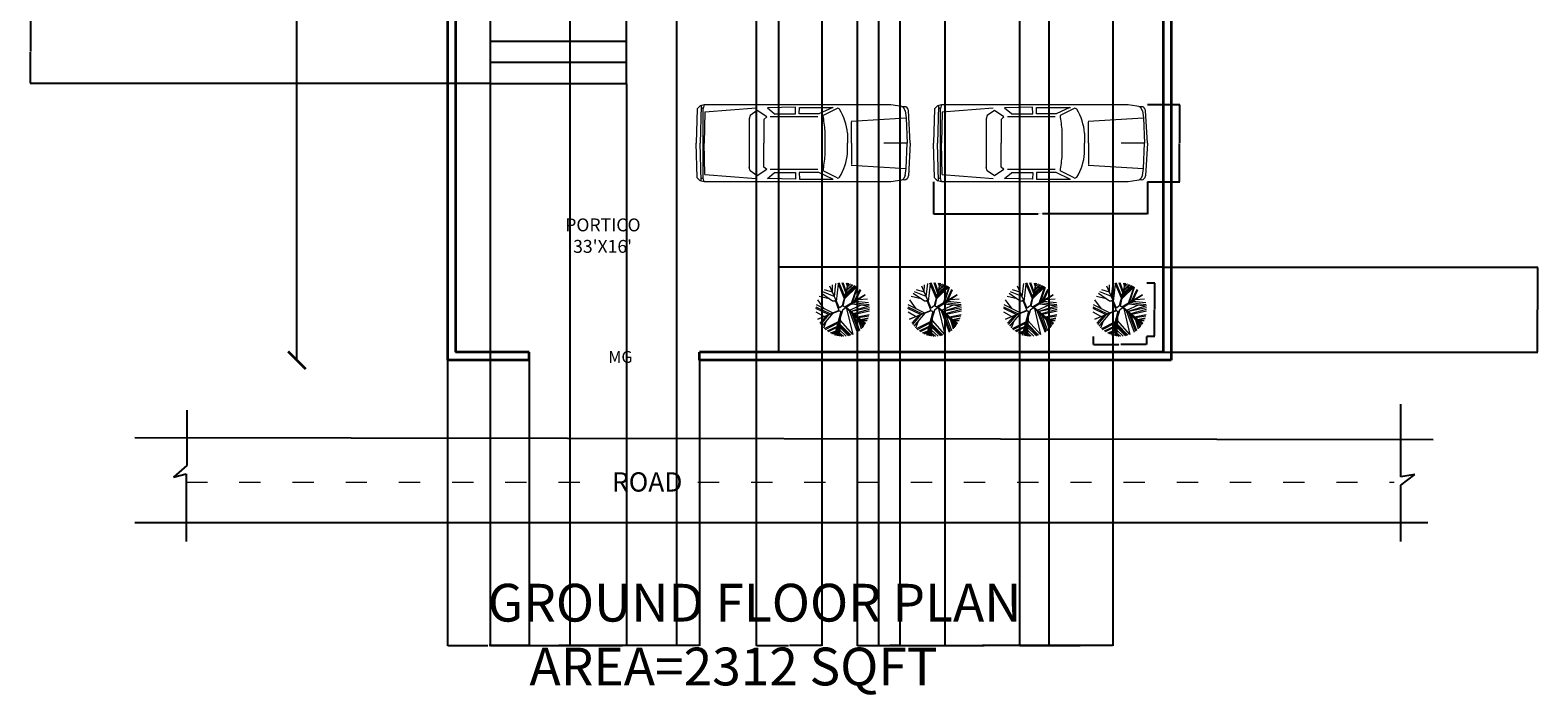
# Model space of a CAD drawing. Units: inches. Extents: x 338 to 1188, y -996 to 127.
# Tile 1 of 15: x 338 to 1188, y -996 to -622. Entities that reach past the tile are written whole.
import ezdxf

# ---------------------------------------------------------------- set-up
doc = ezdxf.new("R2010")
doc.units = ezdxf.units.IN
doc.header["$MEASUREMENT"] = 0
doc.linetypes.add('ACAD_ISO03W100', pattern=[30, 12, -18])
for name, color, linetype, lineweight in [('A-ANNO-DIMS', 5, 'Continuous', 18), ('A-ANNO-TEXT', 7, 'Continuous', 18), ('A-ANNO-TITL', 7, 'Continuous', 35), ('A-AREA-IDEN', 8, 'Continuous', 18), ('A-FLOR-STRS', 7, 'Continuous', 25), ('C-PKNG-VEHI', 8, 'Continuous', 18), ('C-PROP', 1, 'Continuous', 35), ('C-ROAD', 7, 'Continuous', 25), ('C-ROAD-MRKG', 7, 'ACAD_ISO03W100', 18), ('L-PLNT-BEDS', 90, 'Continuous', 25)]:
    doc.layers.add(name, color=color, linetype=linetype, lineweight=lineweight)
doc.layers.add('GRASS', color=90, linetype='Continuous', lineweight=18, transparency=0.7)
doc.styles.get("Standard").update_dxf_attribs({"font": 'arial.ttf'})
doc.dimstyles.get("Standard").update_dxf_attribs({"dimtxt": 0.18, "dimasz": 0.18, "dimexe": 0.18, "dimexo": 0.0625, "dimgap": 0.09, "dimtad": 0, "dimtih": 1, "dimtoh": 1, "dimdec": 1, "dimzin": 0, "dimdsep": 46, "dimlunit": 4, "dimtxsty": 'Standard', "dimcen": 0.09, "dimadec": 0, "dimazin": 0, "dimtfac": 1, "dimtdec": 1, "dimtofl": 0, "dimtmove": 0, "dimatfit": 3, "dimfxl": 1, "dimtolj": 1, "dimtzin": 0, "dimarcsym": 0})

# ---------------------------------------------------------------- blocks, each defined once
blk = doc.blocks.new('A$C4FA53466')
at = {"color": 0}
for p, q in [((0.505, 1.347), (0.266, 1.426)), ((0.717, 0.864), (0.422, 1.538)), ((0.501, 1.356), (0.505, 1.578)), ((0.563, 1.216), (0.612, 1.614)), ((0.627, 1.07), (0.687, 1.601)), ((0.867, 1.166), (0.675, 1.628)), ((0.882, 1.223), (0.709, 1.633)), ((0.91, 1.328), (0.802, 1.64)), ((0.988, 1.623), (0.804, 0.931)), ((0.925, 1.384), (0.834, 1.64)), ((0.836, 0.927), (0.988, 1.623)), ((0.887, 1.159), (1.256, 1.515)), ((0.901, 1.223), (1.228, 1.532)), ((0.914, 1.283), (1.197, 1.549)), ((0.922, 1.323), (1.176, 1.559)), ((0.964, 1.534), (0.938, 1.632)), ((0.938, 1.393), (1.132, 1.579)), ((0.945, 1.425), (1.104, 1.59)), ((0.967, 1.545), (0.952, 1.63)), ((0.965, 1.517), (1.059, 1.605)), ((0.974, 1.559), (1.002, 1.62)), ((1.085, 1.015), (1.262, 1.512)), ((1.121, 1.036), (1.274, 1.503)), ((1.18, 1.071), (1.349, 1.447)), ((1.222, 1.096), (1.37, 1.428)), ((0.501, 0.716), (0.012, 0.965)), ((0.255, 0.841), (0.055, 1.116)), ((0.406, 1.148), (0.102, 1.217)), ((0.506, 1.079), (0.165, 1.314)), ((0.562, 1.217), (0.205, 1.363)), ((0.614, 1.092), (0.506, 1.079)), ((0.604, 1.069), (0.506, 1.079)), ((0.715, 0.784), (0.604, 1.069)), ((0.804, 0.931), (0.717, 0.864)), ((0.879, 0.894), (0.836, 0.927)), ((1.509, 1.265), (0.879, 0.894)), ((0.926, 0.889), (1.509, 1.265)), ((1.03, 0.802), (1.392, 0.963)), ((1.073, 0.767), (1.614, 0.936)), ((1.097, 0.999), (1.632, 0.934)), ((1.148, 1.032), (1.626, 0.972)), ((1.211, 1.073), (1.612, 1.034)), ((1.3, 1.13), (1.573, 1.147)), ((0.384, 0.667), (0, 0.848)), ((0.436, 0.689), (0.003, 0.892)), ((0.237, 0.605), (0.004, 0.735)), ((0.053, 0.528), (0.708, 0.803)), ((0.716, 0.781), (0.053, 0.528)), ((0.321, 0.63), (0.115, 0.4)), ((0.387, 0.655), (0.137, 0.366)), ((0.516, 0.704), (0.179, 0.309)), ((0.313, 0.466), (0.232, 0.248)), ((0.82, 0.82), (0.575, 0.037)), ((0.575, 0.037), (0.769, 0.772)), ((0.732, 0.539), (0.664, 0.015)), ((0.737, 0.554), (0.691, 0.01)), ((0.715, 0.784), (0.775, 0.767)), ((0.744, 0.569), (0.717, 0.006)), ((0.74, 0.488), (1.121, 0.057)), ((0.82, 0.82), (0.904, 0.875)), ((1.521, 0.394), (0.904, 0.875)), ((0.926, 0.889), (1.521, 0.394)), ((0.938, 0.848), (1.126, 0.059)), ((1.016, 0.788), (1.263, 0.13)), ((1.04, 0.769), (1.475, 0.326)), ((1.06, 0.754), (1.5, 0.362)), ((1.081, 0.769), (1.638, 0.886)), ((1.083, 0.725), (1.298, 0.153)), ((1.153, 0.701), (1.64, 0.826)), ((1.161, 0.646), (1.335, 0.182)), ((1.185, 0.674), (1.639, 0.776)), ((1.273, 0.601), (1.627, 0.672)), ((1.298, 0.58), (1.618, 0.629)), ((1.301, 0.503), (1.386, 0.227)), ((1.376, 0.515), (1.599, 0.562)), ((1.392, 0.502), (1.593, 0.545)), ((1.412, 0.486), (1.569, 0.486)), ((0.682, 0.44), (0.255, 0.225)), ((0.673, 0.407), (0.281, 0.201)), ((0.645, 0.301), (0.342, 0.153)), ((0.636, 0.267), (0.375, 0.133)), ((0.608, 0.161), (0.439, 0.093)), ((0.6, 0.133), (0.475, 0.076)), ((0.59, 0.094), (0.501, 0.064)), ((0.701, 0.44), (0.621, 0.024)), ((0.72, 0.07), (0.793, 0)), ((0.722, 0.111), (0.842, 0)), ((0.726, 0.192), (0.924, 0.006)), ((0.73, 0.277), (0.998, 0.019)), ((0.733, 0.326), (1.037, 0.029)), ((0.735, 0.369), (1.067, 0.038)), ((1.365, 0.438), (1.42, 0.26)), ((1.413, 0.39), (1.444, 0.288))]:
    blk.add_line(p, q, dxfattribs=at)
blk = doc.blocks.new('02PCAR12')
at = {"color": 0, "linetype": 'ByBlock'}
for p, q in [((-210, 34), (-211, 0)), ((-207, 37), (-210, 34)), ((-203, 38), (-207, 37)), ((-206, 37), (-207, 0)), ((-204, 34.1), (-206, 35.1)), ((-203, 38.1), (-204, 34.1)), ((-204, -34), (-204, 34)), ((-19, 38), (-203, 38)), ((-202.4, 30.8), (-203, 0)), ((-202.4, 30.8), (-152, 35)), ((-150.8, 32.3), (-157.9, 27.3)), ((-141.5, 26), (-150.8, 32.3)), ((-113.2, 35.5), (-140.8, 34.9)), ((-140.8, 34.9), (-134, 29.2)), ((-113, 29), (-113.2, 35.5)), ((-109.4, 29), (-109.2, 35.3)), ((-109.2, 35.3), (-75.9, 35.3)), ((-76.4, 35.3), (-90, 29)), ((-72.1, 34.2), (-85.9, 27.4)), ((-6, 36), (-19, 38)), ((-5, 32), (-6.4, 34.9)), ((-5, 32), (-4, 25)), ((0, 0), (-1.8, 32.2)), ((-157.9, 27.3), (-158.9, 24.1)), ((-158.9, 24.1), (-158.9, -24)), ((-141.5, 26), (-144.2, 23.5)), ((-144.2, 23.5), (-144.2, 0)), ((-91, 26), (-138, 26)), ((-134, 29), (-113, 29)), ((-90, 29), (-109.4, 29)), ((-58.3, 21.8), (-4, 25)), ((-58, 0), (-58, 21)), ((-4, 25), (-3, 0)), ((-210, -34), (-211, 0)), ((-206, -37), (-207, 0)), ((-202.4, -30.8), (-203, 0)), ((-144.2, -23.5), (-144.2, 0)), ((-84, -12), (-84, 12)), ((-62, 10), (-62, 0)), ((-62, -10), (-62, 0)), ((-58, 0), (-58, -21)), ((-3, 0), (-26, 0)), ((-4, -25), (-3, 0)), ((0, 0), (-1.8, -32.2)), ((-157.9, -27.3), (-158.9, -24.1)), ((-150.8, -32.3), (-157.9, -27.3)), ((-141.5, -26), (-150.8, -32.3)), ((-141.5, -26), (-144.2, -23.5)), ((-140.8, -34.9), (-134, -29.2)), ((-91, -26), (-138, -26)), ((-134, -29), (-113, -29)), ((-113, -29), (-113.2, -35.5)), ((-90, -29), (-109.4, -29)), ((-109.4, -29), (-109.2, -35.3)), ((-76.4, -35.3), (-90, -29)), ((-72.1, -34.2), (-85.9, -27.4)), ((-58.3, -21.8), (-4, -25)), ((-5, -32), (-4, -25)), ((-207, -37), (-210, -34)), ((-203, -38), (-207, -37)), ((-204, -34), (-206, -35)), ((-203, -38), (-204, -34)), ((-19, -38), (-203, -38)), ((-202.4, -30.7), (-152, -34.9)), ((-113.2, -35.5), (-140.8, -34.9)), ((-109.2, -35.3), (-75.9, -35.3)), ((-6, -36), (-19, -38)), ((-5, -32), (-6.4, -34.9))]:
    blk.add_line(p, q, dxfattribs=at)
for centre, radius, start, end in [((-71.4, 32.4), 2, 31.5638, 113.1257), ((-115.3, 5.4), 53.6, 4.9379, 31.5638), ((-8.2, 34), 2, 26.5651, 90), ((-5.8, 32), 4, 3.0128, 90), ((-461, -27.1), 379.1, 5.9264, 8.267), ((-461, 27.1), 379.1, 351.733, 354.0736), ((-115.3, -5.4), 53.6, 328.4362, 355.0621), ((-71.4, -32.4), 2, 246.8743, 328.4362), ((-8.2, -34), 2, 270, 333.4349), ((-5.8, -32), 4, 270, 356.9872)]:
    blk.add_arc(centre, radius, start, end, dxfattribs=at)
blk = doc.blocks.new('_ArchTick')
at = {"color": 0, "linetype": 'ByBlock', "const_width": 0.15}
blk.add_lwpolyline([(-0.5, -0.5), (0.5, 0.5)], dxfattribs=at)
blk = doc.blocks.new('*D7')
at = {"layer": 'A-ANNO-DIMS', "color": 0, "lineweight": -2, "transparency": 16777216}
for p, q in [((488.01, 8.27), (488.01, -388.07)), ((488.01, -807.73), (488.01, -411.39))]:
    blk.add_line(p, q, dxfattribs=at)
at = {"layer": 'Defpoints', "color": 0, "transparency": 16777216}
for p in [(572.96, 8.27), (488.01, -807.73), (572.96, -807.73)]:
    blk.add_point(p, dxfattribs=at)
at = {"layer": 'A-ANNO-DIMS', "color": 0, "lineweight": -2, "transparency": 16777216, "xscale": 10, "yscale": 10, "zscale": 10}
for p, rotation in [((488.01, 8.27), 90), ((488.01, -807.73), 270)]:
    blk.add_blockref('_ArchTick', p, dxfattribs=dict(at, rotation=rotation))
at = {"layer": 'A-ANNO-DIMS', "color": 0, "transparency": 16777216, "insert": (488.01, -399.73), "char_height": 9, "attachment_point": 5, "rotation": 90}
blk.add_mtext("\\A1;68'", dxfattribs=at)
blk = doc.blocks.new('*D11')
at = {"layer": 'A-ANNO-DIMS', "color": 0, "lineweight": -2, "transparency": 16777216}
for p, q in [((967.16, -764.04), (971.81, -764.04)), ((971.63, -764.22), (971.63, -778.96)), ((971.63, -794.07), (971.63, -779.33)), ((967.16, -794.25), (971.81, -794.25))]:
    blk.add_line(p, q, dxfattribs=at)
at = {"layer": 'A-ANNO-DIMS', "color": 0, "transparency": 16777216}
for points in [[(971.6, -764.22), (971.66, -764.22), (971.63, -764.04)], [(971.6, -794.07), (971.66, -794.07), (971.63, -794.25)]]:
    blk.add_solid(points, dxfattribs=at)
at = {"layer": 'Defpoints', "color": 0, "transparency": 16777216}
for p in [(967.1, -764.04), (971.63, -764.04), (967.1, -794.25)]:
    blk.add_point(p, dxfattribs=at)
at = {"layer": 'A-ANNO-DIMS', "color": 0, "transparency": 16777216, "insert": (971.63, -779.14), "char_height": 0.18, "attachment_point": 5}
blk.add_mtext('\\A1;SHRUB 2\'-6" TYP.', dxfattribs=at)
blk = doc.blocks.new('*D12')
at = {"layer": 'A-ANNO-DIMS', "color": 0, "lineweight": -2, "transparency": 16777216}
for p, q in [((936.89, -794.31), (936.89, -798.96)), ((937.07, -798.78), (951.36, -798.78)), ((966.92, -798.78), (952.64, -798.78)), ((967.1, -794.31), (967.1, -798.96))]:
    blk.add_line(p, q, dxfattribs=at)
at = {"layer": 'A-ANNO-DIMS', "color": 0, "transparency": 16777216}
for points in [[(937.07, -798.75), (937.07, -798.81), (936.89, -798.78)], [(966.92, -798.75), (966.92, -798.81), (967.1, -798.78)]]:
    blk.add_solid(points, dxfattribs=at)
at = {"layer": 'Defpoints', "color": 0, "transparency": 16777216}
for p in [(936.89, -794.25), (967.1, -794.25), (967.1, -798.78)]:
    blk.add_point(p, dxfattribs=at)
at = {"layer": 'A-ANNO-DIMS', "color": 0, "transparency": 16777216, "insert": (952, -798.78), "char_height": 0.18, "attachment_point": 5}
blk.add_mtext('\\A1;2\'-6" TYP.', dxfattribs=at)
blk = doc.blocks.new('*D13')
at = {"layer": 'A-ANNO-DIMS', "color": 0, "lineweight": -2, "transparency": 16777216}
for p, q in [((846.88, -707.14), (846.88, -725.36)), ((967.54, -707.14), (967.54, -725.36)), ((847.06, -725.18), (905.99, -725.18)), ((967.36, -725.18), (908.43, -725.18))]:
    blk.add_line(p, q, dxfattribs=at)
at = {"layer": 'A-ANNO-DIMS', "color": 0, "transparency": 16777216}
for points in [[(847.06, -725.15), (847.06, -725.21), (846.88, -725.18)], [(967.36, -725.15), (967.36, -725.21), (967.54, -725.18)]]:
    blk.add_solid(points, dxfattribs=at)
at = {"layer": 'Defpoints', "color": 0, "transparency": 16777216}
for p in [(846.88, -707.08), (967.54, -707.08), (967.54, -725.18)]:
    blk.add_point(p, dxfattribs=at)
at = {"layer": 'A-ANNO-DIMS', "color": 0, "transparency": 16777216, "insert": (907.21, -725.18), "char_height": 0.18, "attachment_point": 5}
blk.add_mtext('\\A1;CAR 10\'-0 1/2" TYP.', dxfattribs=at)
blk = doc.blocks.new('*D14')
at = {"layer": 'A-ANNO-DIMS', "color": 0, "lineweight": -2, "transparency": 16777216}
for p, q in [((967.6, -663.57), (985.82, -663.57)), ((985.64, -663.75), (985.64, -685.14)), ((985.64, -706.9), (985.64, -685.51)), ((967.6, -707.08), (985.82, -707.08))]:
    blk.add_line(p, q, dxfattribs=at)
at = {"layer": 'A-ANNO-DIMS', "color": 0, "transparency": 16777216}
for points in [[(985.61, -663.75), (985.67, -663.75), (985.64, -663.57)], [(985.61, -706.9), (985.67, -706.9), (985.64, -707.08)]]:
    blk.add_solid(points, dxfattribs=at)
at = {"layer": 'Defpoints', "color": 0, "transparency": 16777216}
for p in [(967.54, -663.57), (985.64, -663.57), (967.54, -707.08)]:
    blk.add_point(p, dxfattribs=at)
at = {"layer": 'A-ANNO-DIMS', "color": 0, "transparency": 16777216, "insert": (985.64, -685.32), "char_height": 0.18, "attachment_point": 5}
blk.add_mtext('\\A1;3\'-7 1/2" TYP.', dxfattribs=at)
blk = doc.blocks.new('*D21')
at = {"layer": 'A-ANNO-DIMS', "color": 0, "lineweight": -2, "transparency": 16777216}
for p, q in [((618.97, -807.8), (618.97, -968.86)), ((714.97, -807.8), (714.97, -968.86)), ((619.15, -968.68), (666.64, -968.68)), ((714.79, -968.68), (667.3, -968.68))]:
    blk.add_line(p, q, dxfattribs=at)
at = {"layer": 'A-ANNO-DIMS', "color": 0, "transparency": 16777216}
for points in [[(619.15, -968.65), (619.15, -968.71), (618.97, -968.68)], [(714.79, -968.65), (714.79, -968.71), (714.97, -968.68)]]:
    blk.add_solid(points, dxfattribs=at)
at = {"layer": 'Defpoints', "color": 0, "transparency": 16777216}
for p in [(618.97, -807.73), (714.97, -807.73), (714.97, -968.68)]:
    blk.add_point(p, dxfattribs=at)
at = {"layer": 'A-ANNO-DIMS', "color": 0, "transparency": 16777216, "insert": (666.97, -968.68), "char_height": 0.18, "attachment_point": 5}
blk.add_mtext('\\A1;8\'-0"', dxfattribs=at)
blk = doc.blocks.new('*D22')
at = {"layer": 'A-ANNO-DIMS', "color": 0, "lineweight": -2, "transparency": 16777216}
for p, q in [((596.9, -615.73), (337.66, -615.73)), ((337.84, -615.91), (337.84, -633.55)), ((337.84, -651.55), (337.84, -633.92)), ((596.9, -651.73), (337.66, -651.73))]:
    blk.add_line(p, q, dxfattribs=at)
at = {"layer": 'A-ANNO-DIMS', "color": 0, "transparency": 16777216}
for points in [[(337.81, -615.91), (337.87, -615.91), (337.84, -615.73)], [(337.81, -651.55), (337.87, -651.55), (337.84, -651.73)]]:
    blk.add_solid(points, dxfattribs=at)
at = {"layer": 'Defpoints', "color": 0, "transparency": 16777216}
for p in [(596.96, -615.73), (337.84, -651.73), (596.96, -651.73)]:
    blk.add_point(p, dxfattribs=at)
at = {"layer": 'A-ANNO-DIMS', "color": 0, "transparency": 16777216, "insert": (337.84, -633.73), "char_height": 0.18, "attachment_point": 5}
blk.add_mtext('\\A1;3\'-0"', dxfattribs=at)
blk = doc.blocks.new('*D23')
at = {"layer": 'A-ANNO-DIMS', "color": 0, "lineweight": -2, "transparency": 16777216}
for p, q in [((596.96, -651.8), (596.96, -968.86)), ((673.79, -651.8), (673.79, -968.86)), ((597.14, -968.68), (635.05, -968.68)), ((673.61, -968.68), (635.71, -968.68))]:
    blk.add_line(p, q, dxfattribs=at)
at = {"layer": 'A-ANNO-DIMS', "color": 0, "transparency": 16777216}
for points in [[(597.14, -968.65), (597.14, -968.71), (596.96, -968.68)], [(673.61, -968.65), (673.61, -968.71), (673.79, -968.68)]]:
    blk.add_solid(points, dxfattribs=at)
at = {"layer": 'Defpoints', "color": 0, "transparency": 16777216}
for p in [(596.96, -651.73), (673.79, -651.73), (673.79, -968.68)]:
    blk.add_point(p, dxfattribs=at)
at = {"layer": 'A-ANNO-DIMS', "color": 0, "transparency": 16777216, "insert": (635.38, -968.68), "char_height": 0.18, "attachment_point": 5}
blk.add_mtext('\\A1;6\'-5"', dxfattribs=at)
blk = doc.blocks.new('*D26')
at = {"layer": 'A-ANNO-DIMS', "color": 0, "lineweight": -2, "transparency": 16777216}
for p, q in [((815.96, -297.8), (815.96, -968.86)), ((827.96, -297.8), (827.96, -968.86)), ((816.14, -968.68), (821.64, -968.68)), ((827.78, -968.68), (822.28, -968.68))]:
    blk.add_line(p, q, dxfattribs=at)
at = {"layer": 'A-ANNO-DIMS', "color": 0, "transparency": 16777216}
for points in [[(816.14, -968.65), (816.14, -968.71), (815.96, -968.68)], [(827.78, -968.65), (827.78, -968.71), (827.96, -968.68)]]:
    blk.add_solid(points, dxfattribs=at)
at = {"layer": 'Defpoints', "color": 0, "transparency": 16777216}
for p in [(815.96, -297.73), (827.96, -297.73), (827.96, -968.68)]:
    blk.add_point(p, dxfattribs=at)
at = {"layer": 'A-ANNO-DIMS', "color": 0, "transparency": 16777216, "insert": (821.96, -968.68), "char_height": 0.18, "attachment_point": 5}
blk.add_mtext('\\A1;1\'-0"', dxfattribs=at)
blk = doc.blocks.new('*D27')
at = {"layer": 'A-ANNO-DIMS', "color": 0, "lineweight": -2, "transparency": 16777216}
for p, q in [((911.96, -297.8), (911.96, -968.86)), ((947.96, -297.8), (947.96, -968.86)), ((912.14, -968.68), (929.63, -968.68)), ((947.78, -968.68), (930.29, -968.68))]:
    blk.add_line(p, q, dxfattribs=at)
at = {"layer": 'A-ANNO-DIMS', "color": 0, "transparency": 16777216}
for points in [[(912.14, -968.65), (912.14, -968.71), (911.96, -968.68)], [(947.78, -968.65), (947.78, -968.71), (947.96, -968.68)]]:
    blk.add_solid(points, dxfattribs=at)
at = {"layer": 'Defpoints', "color": 0, "transparency": 16777216}
for p in [(911.96, -297.73), (947.96, -297.73), (947.96, -968.68)]:
    blk.add_point(p, dxfattribs=at)
at = {"layer": 'A-ANNO-DIMS', "color": 0, "transparency": 16777216, "insert": (929.96, -968.68), "char_height": 0.18, "attachment_point": 5}
blk.add_mtext('\\A1;3\'-0"', dxfattribs=at)
blk = doc.blocks.new('*D28')
at = {"layer": 'A-ANNO-DIMS', "color": 0, "lineweight": -2, "transparency": 16777216}
for p, q in [((803.96, -265.8), (803.96, -968.86)), ((947.96, -297.8), (947.96, -968.86)), ((804.14, -968.68), (875.57, -968.68)), ((947.78, -968.68), (876.35, -968.68))]:
    blk.add_line(p, q, dxfattribs=at)
at = {"layer": 'A-ANNO-DIMS', "color": 0, "transparency": 16777216}
for points in [[(804.14, -968.65), (804.14, -968.71), (803.96, -968.68)], [(947.78, -968.65), (947.78, -968.71), (947.96, -968.68)]]:
    blk.add_solid(points, dxfattribs=at)
at = {"layer": 'Defpoints', "color": 0, "transparency": 16777216}
for p in [(803.96, -265.73), (947.96, -297.73), (947.96, -968.68)]:
    blk.add_point(p, dxfattribs=at)
at = {"layer": 'A-ANNO-DIMS', "color": 0, "transparency": 16777216, "insert": (875.96, -968.68), "char_height": 0.18, "attachment_point": 5}
blk.add_mtext('\\A1;12\'-0"', dxfattribs=at)
blk = doc.blocks.new('*D31')
at = {"layer": 'A-ANNO-DIMS', "color": 0, "lineweight": -2, "transparency": 16777216}
for p, q in [((641.96, -149.3), (641.96, -968.86)), ((701.96, -149.3), (701.96, -968.86)), ((642.14, -968.68), (671.63, -968.68)), ((701.78, -968.68), (672.29, -968.68))]:
    blk.add_line(p, q, dxfattribs=at)
at = {"layer": 'A-ANNO-DIMS', "color": 0, "transparency": 16777216}
for points in [[(642.14, -968.65), (642.14, -968.71), (641.96, -968.68)], [(701.78, -968.65), (701.78, -968.71), (701.96, -968.68)]]:
    blk.add_solid(points, dxfattribs=at)
at = {"layer": 'Defpoints', "color": 0, "transparency": 16777216}
for p in [(641.96, -149.23), (701.96, -149.23), (701.96, -968.68)]:
    blk.add_point(p, dxfattribs=at)
at = {"layer": 'A-ANNO-DIMS', "color": 0, "transparency": 16777216, "insert": (671.96, -968.68), "char_height": 0.18, "attachment_point": 5}
blk.add_mtext('\\A1;5\'-0"', dxfattribs=at)
blk = doc.blocks.new('*D35')
at = {"layer": 'A-ANNO-DIMS', "color": 0, "lineweight": -2, "transparency": 16777216}
for p, q in [((572.96, -807.8), (572.96, -968.86)), ((618.97, -807.8), (618.97, -968.86)), ((573.14, -968.68), (595.57, -968.68)), ((618.79, -968.68), (596.37, -968.68))]:
    blk.add_line(p, q, dxfattribs=at)
at = {"layer": 'A-ANNO-DIMS', "color": 0, "transparency": 16777216}
for points in [[(573.14, -968.65), (573.14, -968.71), (572.96, -968.68)], [(618.79, -968.65), (618.79, -968.71), (618.97, -968.68)]]:
    blk.add_solid(points, dxfattribs=at)
at = {"layer": 'Defpoints', "color": 0, "transparency": 16777216}
for p in [(572.96, -807.73), (618.97, -807.73), (618.97, -968.68)]:
    blk.add_point(p, dxfattribs=at)
at = {"layer": 'A-ANNO-DIMS', "color": 0, "transparency": 16777216, "insert": (595.97, -968.68), "char_height": 0.18, "attachment_point": 5}
blk.add_mtext('\\A1;3\'-10"', dxfattribs=at)
blk = doc.blocks.new('*D36')
at = {"layer": 'A-ANNO-DIMS', "color": 0, "lineweight": -2, "transparency": 16777216}
for p, q in [((976.53, -755.23), (1187.6, -755.23)), ((1187.42, -755.41), (1187.42, -779.05)), ((1187.42, -803.05), (1187.42, -779.41)), ((976.53, -803.23), (1187.6, -803.23))]:
    blk.add_line(p, q, dxfattribs=at)
at = {"layer": 'A-ANNO-DIMS', "color": 0, "transparency": 16777216}
for points in [[(1187.39, -755.41), (1187.45, -755.41), (1187.42, -755.23)], [(1187.39, -803.05), (1187.45, -803.05), (1187.42, -803.23)]]:
    blk.add_solid(points, dxfattribs=at)
at = {"layer": 'Defpoints', "color": 0, "transparency": 16777216}
for p in [(976.46, -755.23), (976.46, -803.23), (1187.42, -803.23)]:
    blk.add_point(p, dxfattribs=at)
at = {"layer": 'A-ANNO-DIMS', "color": 0, "transparency": 16777216, "insert": (1187.42, -779.23), "char_height": 0.18, "attachment_point": 5}
blk.add_mtext('\\A1;4\'-0"', dxfattribs=at)
blk = doc.blocks.new('*D42')
at = {"layer": 'A-ANNO-DIMS', "color": 0, "lineweight": -2, "transparency": 16777216}
for p, q in [((746.96, -54.8), (746.96, -968.86)), ((783.89, -54.8), (783.89, -968.86)), ((747.14, -968.68), (765.1, -968.68)), ((783.71, -968.68), (765.76, -968.68))]:
    blk.add_line(p, q, dxfattribs=at)
at = {"layer": 'A-ANNO-DIMS', "color": 0, "transparency": 16777216}
for points in [[(747.14, -968.65), (747.14, -968.71), (746.96, -968.68)], [(783.71, -968.65), (783.71, -968.71), (783.89, -968.68)]]:
    blk.add_solid(points, dxfattribs=at)
at = {"layer": 'Defpoints', "color": 0, "transparency": 16777216}
for p in [(746.96, -54.73), (783.89, -54.73), (783.89, -968.68)]:
    blk.add_point(p, dxfattribs=at)
at = {"layer": 'A-ANNO-DIMS', "color": 0, "transparency": 16777216, "insert": (765.43, -968.68), "char_height": 0.18, "attachment_point": 5}
blk.add_mtext('\\A1;3\'-1"', dxfattribs=at)
blk = doc.blocks.new('*D43')
at = {"layer": 'A-ANNO-DIMS', "color": 0, "lineweight": -2, "transparency": 16777216}
for p, q in [((853.28, -53.93), (853.28, -968.86)), ((895.37, -53.93), (895.37, -968.86)), ((853.46, -968.68), (873.99, -968.68)), ((895.19, -968.68), (874.65, -968.68))]:
    blk.add_line(p, q, dxfattribs=at)
at = {"layer": 'A-ANNO-DIMS', "color": 0, "transparency": 16777216}
for points in [[(853.46, -968.65), (853.46, -968.71), (853.28, -968.68)], [(895.19, -968.65), (895.19, -968.71), (895.37, -968.68)]]:
    blk.add_solid(points, dxfattribs=at)
at = {"layer": 'Defpoints', "color": 0, "transparency": 16777216}
for p in [(853.28, -53.87), (895.37, -53.87), (895.37, -968.68)]:
    blk.add_point(p, dxfattribs=at)
at = {"layer": 'A-ANNO-DIMS', "color": 0, "transparency": 16777216, "insert": (874.32, -968.68), "char_height": 0.18, "attachment_point": 5}
blk.add_mtext('\\A1;3\'-6"', dxfattribs=at)
blk = doc.blocks.new('*D44')
at = {"layer": 'A-ANNO-DIMS', "color": 0, "lineweight": -2, "transparency": 16777216}
for p, q in [((895.37, -53.93), (895.37, -968.86)), ((947.96, -54.8), (947.96, -968.86)), ((895.55, -968.68), (921.12, -968.68)), ((947.78, -968.68), (922.21, -968.68))]:
    blk.add_line(p, q, dxfattribs=at)
at = {"layer": 'A-ANNO-DIMS', "color": 0, "transparency": 16777216}
for points in [[(895.55, -968.65), (895.55, -968.71), (895.37, -968.68)], [(947.78, -968.65), (947.78, -968.71), (947.96, -968.68)]]:
    blk.add_solid(points, dxfattribs=at)
at = {"layer": 'Defpoints', "color": 0, "transparency": 16777216}
for p in [(895.37, -53.87), (947.96, -54.73), (947.96, -968.68)]:
    blk.add_point(p, dxfattribs=at)
at = {"layer": 'A-ANNO-DIMS', "color": 0, "transparency": 16777216, "insert": (921.67, -968.68), "char_height": 0.18, "attachment_point": 5}
blk.add_mtext('\\A1;4\'-4 1/2"', dxfattribs=at)
blk = doc.blocks.new('*D47')
at = {"layer": 'A-ANNO-DIMS', "color": 0, "lineweight": -2, "transparency": 16777216}
for p, q in [((759.67, -755.17), (759.67, 67.25)), ((759.85, 67.07), (867.68, 67.07)), ((976.28, 67.07), (868.46, 67.07)), ((976.46, -755.17), (976.46, 67.25))]:
    blk.add_line(p, q, dxfattribs=at)
at = {"layer": 'A-ANNO-DIMS', "color": 0, "transparency": 16777216}
for points in [[(759.85, 67.1), (759.85, 67.04), (759.67, 67.07)], [(976.28, 67.1), (976.28, 67.04), (976.46, 67.07)]]:
    blk.add_solid(points, dxfattribs=at)
at = {"layer": 'Defpoints', "color": 0, "transparency": 16777216}
for p in [(976.46, 67.07), (759.67, -755.23), (976.46, -755.23)]:
    blk.add_point(p, dxfattribs=at)
at = {"layer": 'A-ANNO-DIMS', "color": 0, "transparency": 16777216, "insert": (868.07, 67.07), "char_height": 0.18, "attachment_point": 5}
blk.add_mtext('\\A1;18\'-1"', dxfattribs=at)

msp = doc.modelspace()

# ---------------------------------------------------------------- linework, layer by layer
at = {"layer": 'A-FLOR-STRS'}
for p, q in [((596.96, -615.73), (596.96, -651.73)), ((673.79, -651.73), (673.79, -615.73)), ((596.96, -627.73), (673.79, -627.73)), ((596.96, -639.73), (673.79, -639.73)), ((596.96, -651.73), (673.79, -651.73))]:
    msp.add_line(p, q, dxfattribs=at)
at = {"layer": 'C-PROP'}
for p, q in [((572.96, 8.27), (572.96, -807.73)), ((577.46, 3.77), (577.46, -803.23)), ((976.46, 3.77), (976.46, -803.23)), ((980.96, 8.27), (980.96, -807.73)), ((618.97, -803.23), (577.46, -803.23)), ((618.97, -807.73), (618.97, -803.23)), ((976.46, -803.23), (714.97, -803.23)), ((714.97, -807.73), (714.97, -803.23)), ((618.97, -807.73), (572.96, -807.73)), ((980.96, -807.73), (714.97, -807.73))]:
    msp.add_line(p, q, dxfattribs=at)
at = {"layer": 'C-ROAD'}
for p, q in [((1110.42, -873.56), (1110.42, -832.44)), ((425.84, -835.91), (425.84, -867.12)), ((396.64, -851.34), (1128.62, -852.38)), ((425.84, -867.12), (418.37, -873.68)), ((418.37, -873.68), (425.49, -871.84)), ((425.49, -871.84), (425.49, -909.88)), ((1118.4, -872.2), (1110.42, -873.56)), ((1110.51, -878.25), (1118.4, -872.2)), ((1110.51, -909.88), (1110.51, -878.25)), ((396.64, -899.34), (1125.68, -899.34))]:
    msp.add_line(p, q, dxfattribs=at)
at = {"layer": 'C-ROAD-MRKG'}
for p, q in [((425.49, -876.53), (662.02, -876.53)), ((714.09, -876.53), (1106.71, -876.53))]:
    msp.add_line(p, q, dxfattribs=at)
at = {"layer": 'L-PLNT-BEDS'}
for p in [(976.46, -755.23), (759.67, -803.23)]:
    msp.add_line(p, (759.67, -755.23), dxfattribs=at)

# ---------------------------------------------------------------- block references
at = {"layer": 'C-PKNG-VEHI', "xscale": 0.5718767357715869, "yscale": 0.5718767357715869, "zscale": 0.5718767357715869}
for p in [(833.8, -685.35), (967.54, -685.35)]:
    msp.add_blockref('02PCAR12', p, dxfattribs=at)
at = {"layer": 'GRASS', "xscale": 18.41745235960633, "yscale": 18.41745235960633, "zscale": 18.41745235960633}
for p in [(780.66, -794.25), (832.5, -794.25), (886.54, -794.25), (936.89, -794.25)]:
    msp.add_blockref('A$C4FA53466', p, dxfattribs=at)

# ---------------------------------------------------------------- texts
at = {"layer": 'A-ANNO-TEXT'}
msp.add_text('MG', height=6.652, dxfattribs=at).set_placement((663.59, -809.22))
at = {"layer": 'A-ANNO-TEXT', "insert": (665.65, -870.94), "char_height": 10.889, "attachment_point": 1}
msp.add_mtext_dynamic_manual_height_columns('ROAD', width=44.8037, gutter_width=1.81, heights=[0], dxfattribs=at)
at = {"layer": 'A-ANNO-TITL', "char_height": 21.2807, "attachment_point": 1}
for s, width, insert in [('GROUND FLOOR PLAN', 345.7385, (595.57, -933.84)), ('AREA=2312 SQFT', 263.9184, (619.09, -969.83))]:
    msp.add_mtext_dynamic_manual_height_columns(s, width=width, gutter_width=3.55, heights=[0], dxfattribs=dict(at, insert=insert))
at = {"layer": 'A-AREA-IDEN', "insert": (630.4, -727.78), "char_height": 7.2703, "attachment_point": 1}
msp.add_mtext_dynamic_manual_height_columns("    PORTICO\\P      33'X16'", width=63.7182, gutter_width=1, heights=[0], dxfattribs=at)

# ---------------------------------------------------------------- dimensions: what is measured, and where the dimension line sits
at = {"layer": 'A-ANNO-DIMS'}
for base, p1, p2, picture, middle in [((976.46, 67.07), (759.67, -755.23), (976.46, -755.23), '*D47', (868.07, 67.07)), ((783.89, -968.68), (746.96, -54.73), (783.89, -54.73), '*D42', (765.43, -968.68)), ((895.37, -968.68), (853.28, -53.87), (895.37, -53.87), '*D43', (874.32, -968.68)), ((947.96, -968.68), (895.37, -53.87), (947.96, -54.73), '*D44', (921.67, -968.68)), ((701.96, -968.68), (641.96, -149.23), (701.96, -149.23), '*D31', (671.96, -968.68)), ((947.96, -968.68), (803.96, -265.73), (947.96, -297.73), '*D28', (875.96, -968.68)), ((827.96, -968.68), (815.96, -297.73), (827.96, -297.73), '*D26', (821.96, -968.68)), ((947.96, -968.68), (911.96, -297.73), (947.96, -297.73), '*D27', (929.96, -968.68)), ((673.79, -968.68), (596.96, -651.73), (673.79, -651.73), '*D23', (635.38, -968.68)), ((618.97, -968.68), (572.96, -807.73), (618.97, -807.73), '*D35', (595.97, -968.68)), ((714.97, -968.68), (618.97, -807.73), (714.97, -807.73), '*D21', (666.97, -968.68))]:
    dim = msp.add_linear_dim(base=base, p1=p1, p2=p2, dimstyle='Standard', override={"dimdec": 1, "dimlfac": 1, "dimrnd": 0, "dimzin": 1, "dimdsep": 46, "dimlunit": 4, "dimfrac": 2}, dxfattribs=at)
    dim.commit()
    dim.dimension.update_dxf_attribs({"geometry": picture, "text_midpoint": middle})
for base, p1, p2, override, picture, middle in [((488.01, -807.73), (572.96, 8.27), (572.96, -807.73), {"dimtxt": 9, "dimasz": 10, "dimgap": 4, "dimtad": 0, "dimtih": 0, "dimblk1": 'ArchTick', "dimblk2": 'ArchTick', "dimsah": 1, "dimse1": 1, "dimse2": 1, "dimclrd": 0, "dimclre": 0, "dimclrt": 0}, '*D7', (488.01, -399.73)), ((337.84, -651.73), (596.96, -615.73), (596.96, -651.73), {"dimdec": 1, "dimlfac": 1, "dimrnd": 0, "dimzin": 1, "dimdsep": 46, "dimlunit": 4, "dimfrac": 2}, '*D22', (337.84, -633.73)), ((1187.42, -803.23), (976.46, -755.23), (976.46, -803.23), {"dimdec": 1, "dimlfac": 1, "dimrnd": 0, "dimzin": 1, "dimdsep": 46, "dimlunit": 4, "dimfrac": 2}, '*D36', (1187.42, -779.23))]:
    dim = msp.add_linear_dim(base=base, p1=p1, p2=p2, angle=90, dimstyle='Standard', override=override, dxfattribs=at)
    dim.commit()
    dim.dimension.update_dxf_attribs({"geometry": picture, "text_midpoint": middle})
for base, p1, p2, text, picture, middle in [((985.64, -663.57), (967.54, -707.08), (967.54, -663.57), '<> TYP.', '*D14', (985.64, -685.32)), ((971.63, -764.04), (967.1, -794.25), (967.1, -764.04), 'SHRUB <> TYP.', '*D11', (971.63, -779.14))]:
    dim = msp.add_linear_dim(base=base, p1=p1, p2=p2, angle=90, text=text, dimstyle='Standard', override={"dimdec": 1, "dimlfac": 1, "dimrnd": 0, "dimzin": 1, "dimdsep": 46, "dimlunit": 4, "dimfrac": 2}, dxfattribs=at)
    dim.commit()
    dim.dimension.update_dxf_attribs({"geometry": picture, "text_midpoint": middle})
for base, p1, p2, text, picture, middle in [((967.54, -725.18), (846.88, -707.08), (967.54, -707.08), 'CAR <> TYP.', '*D13', (907.21, -725.18)), ((967.1, -798.78), (936.89, -794.25), (967.1, -794.25), '<> TYP.', '*D12', (952, -798.78))]:
    dim = msp.add_linear_dim(base=base, p1=p1, p2=p2, text=text, dimstyle='Standard', override={"dimdec": 1, "dimlfac": 1, "dimrnd": 0, "dimzin": 1, "dimdsep": 46, "dimlunit": 4, "dimfrac": 2}, dxfattribs=at)
    dim.commit()
    dim.dimension.update_dxf_attribs({"geometry": picture, "text_midpoint": middle})

doc.saveas('drawing.dxf')
